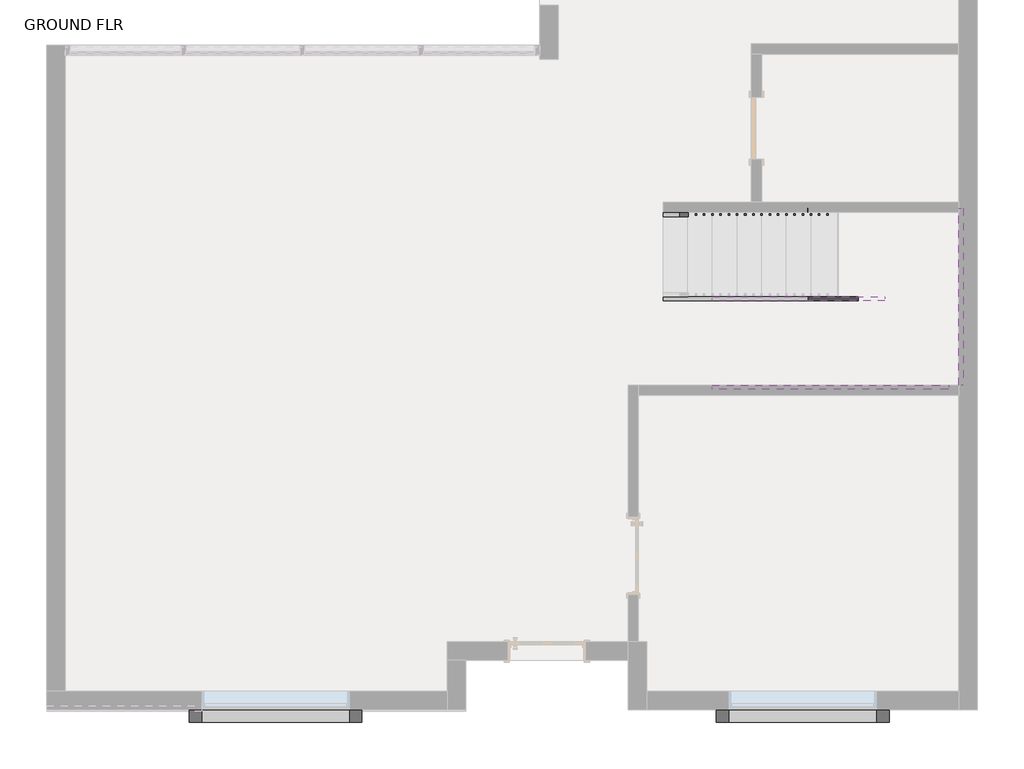
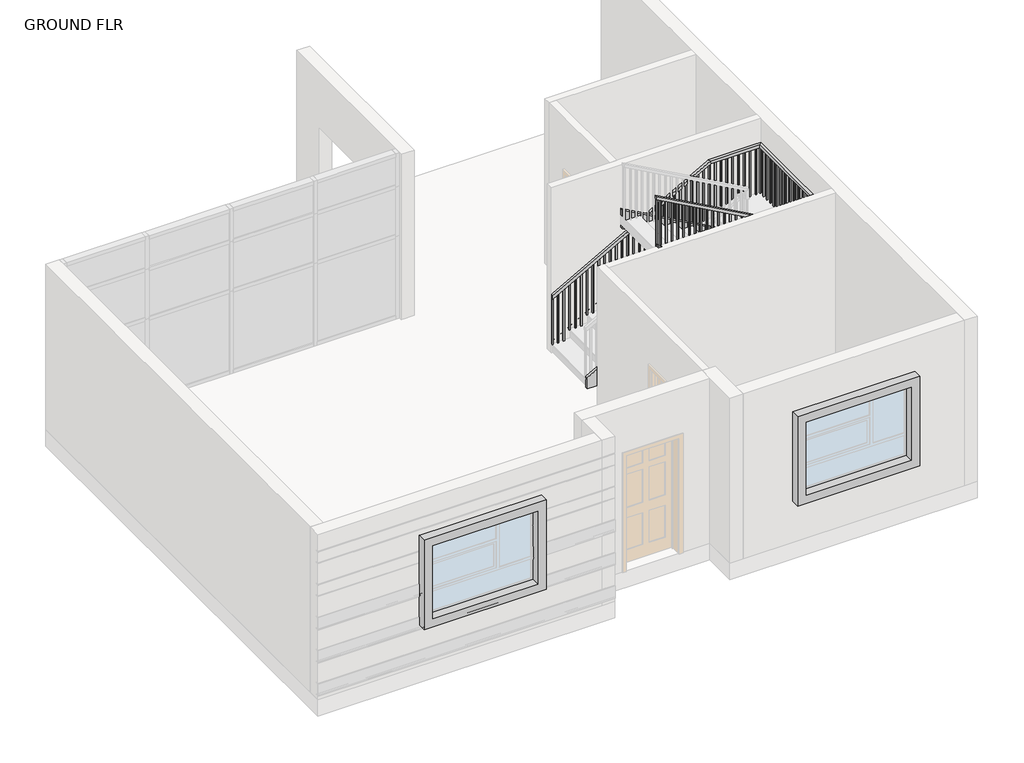
# One storey, part 4 of 4: 5 members, 2 proxies, 1 railing.
"""IFC4 building model written with IfcOpenShell, lengths in millimetres."""

from ifc_helpers import new_model, si_unit, frame, origin, place, context, project, spatial, polyline, outline, extrude, faceted_brep, transform, mapped, element, save
from components import generic_models_3_generic_models_3_1617b94e, generic_models_6_generic_models_3_5dde034f

model = new_model("IFC4")

# Units and contexts
model_context = context("Model", 3, world=origin())
ifc_project = project(units=[si_unit("LENGTHUNIT", "METRE", prefix="MILLI")], contexts=[model_context])

# Site, building, storey
site = spatial("IfcSite", under=ifc_project)
building = spatial("IfcBuilding", under=site)
storey = spatial("IfcBuildingStorey", under=building, Name="GROUND FLR", Elevation=304.8)

# Proxies
placement = place(None, origin())
generic_models_3_generic_models_3_shape = generic_models_3_generic_models_3_1617b94e(model_context)
element("IfcBuildingElementProxy", 1, Name="Generic Models 3 : Generic Models 3", ObjectType="Generic Models 3 : Generic Models 3", at=placement, inside=storey, context=model_context, shape_type="MappedRepresentation", body=[
    mapped(generic_models_3_generic_models_3_shape, transform((0.0, 0.0, 0.0), x_axis=(1.0, 0.0, 0.0), y_axis=(0.0, 1.0, 0.0), z_axis=(0.0, 0.0, 1.0))),
])
generic_models_6_generic_models_3_shape = generic_models_6_generic_models_3_5dde034f(model_context)
element("IfcBuildingElementProxy", 2, Name="Generic Models 6 : Generic Models 3", ObjectType="Generic Models 6 : Generic Models 3", at=placement, inside=storey, context=model_context, shape_type="MappedRepresentation", body=[
    mapped(generic_models_6_generic_models_3_shape, transform((0.0, 0.0, 0.0), x_axis=(1.0, 0.0, 0.0), y_axis=(0.0, 1.0, 0.0), z_axis=(0.0, 0.0, 1.0))),
])

# Members
element("IfcMember", 3, ObjectType="Stringer - 2\" Width", at=placement, inside=storey, context=model_context, shape_type="SweptSolid", body=[
    extrude(outline(polyline([(512.3983948, 1775.9671209), (304.8, 1775.9671209), (304.8, 2029.9116237), (2074.3333333, 5215.0716237), (2074.3333333, 4587.4500103), (512.3983948, 1775.9671209)])), frame((0.0, 3696.9223211, 0.0), z_axis=(0.0, 1.0, 0.0), x_axis=(0.0, 0.0, 1.0)), (0.0, 0.0, 1.0), 50.8),
])
element("IfcMember", 4, ObjectType="Stringer - 2\" Width", at=placement, inside=storey, context=model_context, shape_type="SweptSolid", body=[
    extrude(outline(polyline([(5433.5671209, 3747.7223211), (5484.3671209, 3747.7223211), (5484.3671209, 1563.3223211), (5433.5671209, 1563.3223211), (5433.5671209, 3747.7223211)])), frame((0.0, 0.0, 1769.5333333), z_axis=(0.0, 0.0, 1.0), x_axis=(1.0, 0.0, 0.0)), (0.0, 0.0, 1.0), 304.8),
])
element("IfcMember", 5, ObjectType="Stringer - 2\" Width", at=placement, inside=storey, context=model_context, shape_type="SweptSolid", body=[
    extrude(outline(polyline([(1769.5333333, 5304.3242315), (3391.0650614, 2385.5671209), (3042.3863873, 2385.5671209), (1769.5333333, 4676.7026181), (1769.5333333, 5304.3242315)])), frame((0.0, 1512.5223211, 0.0), z_axis=(0.0, 1.0, 0.0), x_axis=(0.0, 0.0, 1.0)), (0.0, 0.0, 1.0), 50.8),
])
element("IfcMember", 6, ObjectType="Stringer - 2\" Width", at=placement, inside=storey, context=model_context, shape_type="SweptSolid", body=[
    extrude(outline(polyline([(512.3983948, 1775.9671209), (304.8, 1775.9671209), (304.8, 2029.9116237), (1659.4974984, 4468.3671209), (2008.1761726, 4468.3671209), (512.3983948, 1775.9671209)])), frame((0.0, 2604.7223211, 0.0), z_axis=(0.0, 1.0, 0.0), x_axis=(0.0, 0.0, 1.0)), (0.0, 0.0, 1.0), 50.8),
])
element("IfcMember", 7, ObjectType="Stringer - 2\" Width", at=placement, inside=storey, context=model_context, shape_type="SweptSolid", body=[
    extrude(outline(polyline([(1857.053054, 4519.1671209), (2205.7317281, 4519.1671209), (3391.0650614, 2385.5671209), (3042.3863873, 2385.5671209), (1857.053054, 4519.1671209)])), frame((0.0, 2604.7223211, 0.0), z_axis=(0.0, 1.0, 0.0), x_axis=(0.0, 0.0, 1.0)), (0.0, 0.0, 1.0), 50.8),
])

# Railing
element("IfcRailing", 8, ObjectType="Handrail - Rectangular", at=placement, inside=storey, context=model_context, shape_type="SolidModel", body=[
    faceted_brep([(1775.9671209, 3696.9223211, 1388.5333333), (1775.9671209, 3696.9223211, 1330.420221), (1775.9671209, 3646.1223211, 1330.420221), (1775.9671209, 3646.1223211, 1388.5333333), (4519.1671209, 3696.9223211, 2912.5333333), (4532.3307231, 3696.9223211, 2861.7333333), (4532.3307231, 3646.1223211, 2861.7333333), (4519.1671209, 3646.1223211, 2912.5333333), (5433.5671209, 3696.9223211, 2912.5333333), (5433.5671209, 3696.9223211, 2861.7333333), (5382.7671209, 3646.1223211, 2861.7333333), (5382.7671209, 3646.1223211, 2912.5333333), (5433.5671209, 1563.3223211, 2912.5333333), (5433.5671209, 1563.3223211, 2861.7333333), (5382.7671209, 1614.1223211, 2861.7333333), (5382.7671209, 1614.1223211, 2912.5333333), (4823.9671209, 1563.3223211, 2912.5333333), (4810.8035186, 1563.3223211, 2861.7333333), (4810.8035186, 1614.1223211, 2861.7333333), (4823.9671209, 1614.1223211, 2912.5333333), (2385.5671209, 1563.3223211, 4267.2), (2385.5671209, 1614.1223211, 4267.2), (2385.5671209, 1614.1223211, 4209.0868876), (2385.5671209, 1563.3223211, 4209.0868876)], [[[0, 1, 2, 3]], [[1, 0, 4, 5]], [[2, 1, 5, 6]], [[3, 2, 6, 7]], [[0, 3, 7, 4]], [[5, 4, 8, 9]], [[6, 5, 9, 10]], [[7, 6, 10, 11]], [[4, 7, 11, 8]], [[9, 8, 12, 13]], [[10, 9, 13, 14]], [[11, 10, 14, 15]], [[8, 11, 15, 12]], [[13, 12, 16, 17]], [[14, 13, 17, 18]], [[15, 14, 18, 19]], [[12, 15, 19, 16]], [[20, 21, 22, 23]], [[17, 16, 20, 23]], [[18, 17, 23, 22]], [[19, 18, 22, 21]], [[16, 19, 21, 20]]]),
    extrude(outline(polyline([(4172.045221, 2452.2421209), (3183.4666667, 2452.2421209), (3183.4666667, 2471.2921209), (4161.4618876, 2471.2921209), (4172.045221, 2452.2421209)])), frame((0.0, 1579.1973211, 0.0), z_axis=(0.0, 1.0, 0.0), x_axis=(0.0, 0.0, 1.0)), (0.0, 0.0, 1.0), 19.05),
    extrude(outline(polyline([(4115.6007765, 2553.8421209), (3183.4666667, 2553.8421209), (3183.4666667, 2572.8921209), (4105.0174432, 2572.8921209), (4115.6007765, 2553.8421209)])), frame((0.0, 1579.1973211, 0.0), z_axis=(0.0, 1.0, 0.0), x_axis=(0.0, 0.0, 1.0)), (0.0, 0.0, 1.0), 19.05),
    extrude(outline(polyline([(4059.1563321, 2655.4421209), (3183.4666667, 2655.4421209), (3183.4666667, 2674.4921209), (4048.5729988, 2674.4921209), (4059.1563321, 2655.4421209)])), frame((0.0, 1579.1973211, 0.0), z_axis=(0.0, 1.0, 0.0), x_axis=(0.0, 0.0, 1.0)), (0.0, 0.0, 1.0), 19.05),
    extrude(outline(polyline([(4002.7118876, 2757.0421209), (3014.1333333, 2757.0421209), (3014.1333333, 2776.0921209), (3992.1285543, 2776.0921209), (4002.7118876, 2757.0421209)])), frame((0.0, 1579.1973211, 0.0), z_axis=(0.0, 1.0, 0.0), x_axis=(0.0, 0.0, 1.0)), (0.0, 0.0, 1.0), 19.05),
    extrude(outline(polyline([(3946.2674432, 2858.6421209), (3014.1333333, 2858.6421209), (3014.1333333, 2877.6921209), (3935.6841099, 2877.6921209), (3946.2674432, 2858.6421209)])), frame((0.0, 1579.1973211, 0.0), z_axis=(0.0, 1.0, 0.0), x_axis=(0.0, 0.0, 1.0)), (0.0, 0.0, 1.0), 19.05),
    extrude(outline(polyline([(3889.8229988, 2960.2421209), (3014.1333333, 2960.2421209), (3014.1333333, 2979.2921209), (3879.2396654, 2979.2921209), (3889.8229988, 2960.2421209)])), frame((0.0, 1579.1973211, 0.0), z_axis=(0.0, 1.0, 0.0), x_axis=(0.0, 0.0, 1.0)), (0.0, 0.0, 1.0), 19.05),
    extrude(outline(polyline([(3833.3785543, 3061.8421209), (2844.8, 3061.8421209), (2844.8, 3080.8921209), (3822.795221, 3080.8921209), (3833.3785543, 3061.8421209)])), frame((0.0, 1579.1973211, 0.0), z_axis=(0.0, 1.0, 0.0), x_axis=(0.0, 0.0, 1.0)), (0.0, 0.0, 1.0), 19.05),
    extrude(outline(polyline([(3776.9341099, 3163.4421209), (2844.8, 3163.4421209), (2844.8, 3182.4921209), (3766.3507765, 3182.4921209), (3776.9341099, 3163.4421209)])), frame((0.0, 1579.1973211, 0.0), z_axis=(0.0, 1.0, 0.0), x_axis=(0.0, 0.0, 1.0)), (0.0, 0.0, 1.0), 19.05),
    extrude(outline(polyline([(3720.4896654, 3265.0421209), (2844.8, 3265.0421209), (2844.8, 3284.0921209), (3709.9063321, 3284.0921209), (3720.4896654, 3265.0421209)])), frame((0.0, 1579.1973211, 0.0), z_axis=(0.0, 1.0, 0.0), x_axis=(0.0, 0.0, 1.0)), (0.0, 0.0, 1.0), 19.05),
    extrude(outline(polyline([(3664.045221, 3366.6421209), (2675.4666667, 3366.6421209), (2675.4666667, 3385.6921209), (3653.4618876, 3385.6921209), (3664.045221, 3366.6421209)])), frame((0.0, 1579.1973211, 0.0), z_axis=(0.0, 1.0, 0.0), x_axis=(0.0, 0.0, 1.0)), (0.0, 0.0, 1.0), 19.05),
    extrude(outline(polyline([(3607.6007765, 3468.2421209), (2675.4666667, 3468.2421209), (2675.4666667, 3487.2921209), (3597.0174432, 3487.2921209), (3607.6007765, 3468.2421209)])), frame((0.0, 1579.1973211, 0.0), z_axis=(0.0, 1.0, 0.0), x_axis=(0.0, 0.0, 1.0)), (0.0, 0.0, 1.0), 19.05),
    extrude(outline(polyline([(3551.1563321, 3569.8421209), (2675.4666667, 3569.8421209), (2675.4666667, 3588.8921209), (3540.5729988, 3588.8921209), (3551.1563321, 3569.8421209)])), frame((0.0, 1579.1973211, 0.0), z_axis=(0.0, 1.0, 0.0), x_axis=(0.0, 0.0, 1.0)), (0.0, 0.0, 1.0), 19.05),
    extrude(outline(polyline([(3494.7118876, 3671.4421209), (2506.1333333, 3671.4421209), (2506.1333333, 3690.4921209), (3484.1285543, 3690.4921209), (3494.7118876, 3671.4421209)])), frame((0.0, 1579.1973211, 0.0), z_axis=(0.0, 1.0, 0.0), x_axis=(0.0, 0.0, 1.0)), (0.0, 0.0, 1.0), 19.05),
    extrude(outline(polyline([(3438.2674432, 3773.0421209), (2506.1333333, 3773.0421209), (2506.1333333, 3792.0921209), (3427.6841099, 3792.0921209), (3438.2674432, 3773.0421209)])), frame((0.0, 1579.1973211, 0.0), z_axis=(0.0, 1.0, 0.0), x_axis=(0.0, 0.0, 1.0)), (0.0, 0.0, 1.0), 19.05),
    extrude(outline(polyline([(3381.8229988, 3874.6421209), (2506.1333333, 3874.6421209), (2506.1333333, 3893.6921209), (3371.2396654, 3893.6921209), (3381.8229988, 3874.6421209)])), frame((0.0, 1579.1973211, 0.0), z_axis=(0.0, 1.0, 0.0), x_axis=(0.0, 0.0, 1.0)), (0.0, 0.0, 1.0), 19.05),
    extrude(outline(polyline([(3325.3785543, 3976.2421209), (2336.8, 3976.2421209), (2336.8, 3995.2921209), (3314.795221, 3995.2921209), (3325.3785543, 3976.2421209)])), frame((0.0, 1579.1973211, 0.0), z_axis=(0.0, 1.0, 0.0), x_axis=(0.0, 0.0, 1.0)), (0.0, 0.0, 1.0), 19.05),
    extrude(outline(polyline([(3268.9341099, 4077.8421209), (2336.8, 4077.8421209), (2336.8, 4096.8921209), (3258.3507765, 4096.8921209), (3268.9341099, 4077.8421209)])), frame((0.0, 1579.1973211, 0.0), z_axis=(0.0, 1.0, 0.0), x_axis=(0.0, 0.0, 1.0)), (0.0, 0.0, 1.0), 19.05),
    extrude(outline(polyline([(3212.4896654, 4179.4421209), (2336.8, 4179.4421209), (2336.8, 4198.4921209), (3201.9063321, 4198.4921209), (3212.4896654, 4179.4421209)])), frame((0.0, 1579.1973211, 0.0), z_axis=(0.0, 1.0, 0.0), x_axis=(0.0, 0.0, 1.0)), (0.0, 0.0, 1.0), 19.05),
    extrude(outline(polyline([(3156.045221, 4281.0421209), (2167.4666667, 4281.0421209), (2167.4666667, 4300.0921209), (3145.4618876, 4300.0921209), (3156.045221, 4281.0421209)])), frame((0.0, 1579.1973211, 0.0), z_axis=(0.0, 1.0, 0.0), x_axis=(0.0, 0.0, 1.0)), (0.0, 0.0, 1.0), 19.05),
    extrude(outline(polyline([(3099.6007765, 4382.6421209), (2167.4666667, 4382.6421209), (2167.4666667, 4401.6921209), (3089.0174432, 4401.6921209), (3099.6007765, 4382.6421209)])), frame((0.0, 1579.1973211, 0.0), z_axis=(0.0, 1.0, 0.0), x_axis=(0.0, 0.0, 1.0)), (0.0, 0.0, 1.0), 19.05),
    extrude(outline(polyline([(3043.1563321, 4484.2421209), (2167.4666667, 4484.2421209), (2167.4666667, 4503.2921209), (3032.5729988, 4503.2921209), (3043.1563321, 4484.2421209)])), frame((0.0, 1579.1973211, 0.0), z_axis=(0.0, 1.0, 0.0), x_axis=(0.0, 0.0, 1.0)), (0.0, 0.0, 1.0), 19.05),
    extrude(outline(polyline([(2986.7118876, 4585.8421209), (1998.1333333, 4585.8421209), (1998.1333333, 4604.8921209), (2976.1285543, 4604.8921209), (2986.7118876, 4585.8421209)])), frame((0.0, 1579.1973211, 0.0), z_axis=(0.0, 1.0, 0.0), x_axis=(0.0, 0.0, 1.0)), (0.0, 0.0, 1.0), 19.05),
    extrude(outline(polyline([(2930.2674432, 4687.4421209), (1998.1333333, 4687.4421209), (1998.1333333, 4706.4921209), (2919.6841099, 4706.4921209), (2930.2674432, 4687.4421209)])), frame((0.0, 1579.1973211, 0.0), z_axis=(0.0, 1.0, 0.0), x_axis=(0.0, 0.0, 1.0)), (0.0, 0.0, 1.0), 19.05),
    extrude(outline(polyline([(2873.8229988, 4789.0421209), (1998.1333333, 4789.0421209), (1998.1333333, 4808.0921209), (2863.2396654, 4808.0921209), (2873.8229988, 4789.0421209)])), frame((0.0, 1579.1973211, 0.0), z_axis=(0.0, 1.0, 0.0), x_axis=(0.0, 0.0, 1.0)), (0.0, 0.0, 1.0), 19.05),
    extrude(outline(polyline([(4909.6921209, 1579.1973211), (4890.6421209, 1579.1973211), (4890.6421209, 1598.2473211), (4909.6921209, 1598.2473211), (4909.6921209, 1579.1973211)])), frame((0.0, 0.0, 1998.1333333), z_axis=(0.0, 0.0, 1.0), x_axis=(1.0, 0.0, 0.0)), (0.0, 0.0, 1.0), 863.6),
    extrude(outline(polyline([(5011.2921209, 1579.1973211), (4992.2421209, 1579.1973211), (4992.2421209, 1598.2473211), (5011.2921209, 1598.2473211), (5011.2921209, 1579.1973211)])), frame((0.0, 0.0, 1998.1333333), z_axis=(0.0, 0.0, 1.0), x_axis=(1.0, 0.0, 0.0)), (0.0, 0.0, 1.0), 863.6),
    extrude(outline(polyline([(5112.8921209, 1579.1973211), (5093.8421209, 1579.1973211), (5093.8421209, 1598.2473211), (5112.8921209, 1598.2473211), (5112.8921209, 1579.1973211)])), frame((0.0, 0.0, 1998.1333333), z_axis=(0.0, 0.0, 1.0), x_axis=(1.0, 0.0, 0.0)), (0.0, 0.0, 1.0), 863.6),
    extrude(outline(polyline([(5214.4921209, 1579.1973211), (5195.4421209, 1579.1973211), (5195.4421209, 1598.2473211), (5214.4921209, 1598.2473211), (5214.4921209, 1579.1973211)])), frame((0.0, 0.0, 1998.1333333), z_axis=(0.0, 0.0, 1.0), x_axis=(1.0, 0.0, 0.0)), (0.0, 0.0, 1.0), 863.6),
    extrude(outline(polyline([(5316.0921209, 1579.1973211), (5297.0421209, 1579.1973211), (5297.0421209, 1598.2473211), (5316.0921209, 1598.2473211), (5316.0921209, 1579.1973211)])), frame((0.0, 0.0, 1998.1333333), z_axis=(0.0, 0.0, 1.0), x_axis=(1.0, 0.0, 0.0)), (0.0, 0.0, 1.0), 863.6),
    extrude(outline(polyline([(5417.6921209, 1649.0473211), (5417.6921209, 1629.9973211), (5398.6421209, 1629.9973211), (5398.6421209, 1649.0473211), (5417.6921209, 1649.0473211)])), frame((0.0, 0.0, 1998.1333333), z_axis=(0.0, 0.0, 1.0), x_axis=(1.0, 0.0, 0.0)), (0.0, 0.0, 1.0), 863.6),
    extrude(outline(polyline([(5417.6921209, 1750.6473211), (5417.6921209, 1731.5973211), (5398.6421209, 1731.5973211), (5398.6421209, 1750.6473211), (5417.6921209, 1750.6473211)])), frame((0.0, 0.0, 1998.1333333), z_axis=(0.0, 0.0, 1.0), x_axis=(1.0, 0.0, 0.0)), (0.0, 0.0, 1.0), 863.6),
    extrude(outline(polyline([(5417.6921209, 1852.2473211), (5417.6921209, 1833.1973211), (5398.6421209, 1833.1973211), (5398.6421209, 1852.2473211), (5417.6921209, 1852.2473211)])), frame((0.0, 0.0, 1998.1333333), z_axis=(0.0, 0.0, 1.0), x_axis=(1.0, 0.0, 0.0)), (0.0, 0.0, 1.0), 863.6),
    extrude(outline(polyline([(5417.6921209, 1953.8473211), (5417.6921209, 1934.7973211), (5398.6421209, 1934.7973211), (5398.6421209, 1953.8473211), (5417.6921209, 1953.8473211)])), frame((0.0, 0.0, 1998.1333333), z_axis=(0.0, 0.0, 1.0), x_axis=(1.0, 0.0, 0.0)), (0.0, 0.0, 1.0), 863.6),
    extrude(outline(polyline([(5417.6921209, 2055.4473211), (5417.6921209, 2036.3973211), (5398.6421209, 2036.3973211), (5398.6421209, 2055.4473211), (5417.6921209, 2055.4473211)])), frame((0.0, 0.0, 1998.1333333), z_axis=(0.0, 0.0, 1.0), x_axis=(1.0, 0.0, 0.0)), (0.0, 0.0, 1.0), 863.6),
    extrude(outline(polyline([(5417.6921209, 2157.0473211), (5417.6921209, 2137.9973211), (5398.6421209, 2137.9973211), (5398.6421209, 2157.0473211), (5417.6921209, 2157.0473211)])), frame((0.0, 0.0, 1998.1333333), z_axis=(0.0, 0.0, 1.0), x_axis=(1.0, 0.0, 0.0)), (0.0, 0.0, 1.0), 863.6),
    extrude(outline(polyline([(5417.6921209, 2258.6473211), (5417.6921209, 2239.5973211), (5398.6421209, 2239.5973211), (5398.6421209, 2258.6473211), (5417.6921209, 2258.6473211)])), frame((0.0, 0.0, 1998.1333333), z_axis=(0.0, 0.0, 1.0), x_axis=(1.0, 0.0, 0.0)), (0.0, 0.0, 1.0), 863.6),
    extrude(outline(polyline([(5417.6921209, 2360.2473211), (5417.6921209, 2341.1973211), (5398.6421209, 2341.1973211), (5398.6421209, 2360.2473211), (5417.6921209, 2360.2473211)])), frame((0.0, 0.0, 1998.1333333), z_axis=(0.0, 0.0, 1.0), x_axis=(1.0, 0.0, 0.0)), (0.0, 0.0, 1.0), 863.6),
    extrude(outline(polyline([(5417.6921209, 2461.8473211), (5417.6921209, 2442.7973211), (5398.6421209, 2442.7973211), (5398.6421209, 2461.8473211), (5417.6921209, 2461.8473211)])), frame((0.0, 0.0, 1998.1333333), z_axis=(0.0, 0.0, 1.0), x_axis=(1.0, 0.0, 0.0)), (0.0, 0.0, 1.0), 863.6),
    extrude(outline(polyline([(5417.6921209, 2563.4473211), (5417.6921209, 2544.3973211), (5398.6421209, 2544.3973211), (5398.6421209, 2563.4473211), (5417.6921209, 2563.4473211)])), frame((0.0, 0.0, 1998.1333333), z_axis=(0.0, 0.0, 1.0), x_axis=(1.0, 0.0, 0.0)), (0.0, 0.0, 1.0), 863.6),
    extrude(outline(polyline([(5417.6921209, 2665.0473211), (5417.6921209, 2645.9973211), (5398.6421209, 2645.9973211), (5398.6421209, 2665.0473211), (5417.6921209, 2665.0473211)])), frame((0.0, 0.0, 1998.1333333), z_axis=(0.0, 0.0, 1.0), x_axis=(1.0, 0.0, 0.0)), (0.0, 0.0, 1.0), 863.6),
    extrude(outline(polyline([(5417.6921209, 2766.6473211), (5417.6921209, 2747.5973211), (5398.6421209, 2747.5973211), (5398.6421209, 2766.6473211), (5417.6921209, 2766.6473211)])), frame((0.0, 0.0, 1998.1333333), z_axis=(0.0, 0.0, 1.0), x_axis=(1.0, 0.0, 0.0)), (0.0, 0.0, 1.0), 863.6),
    extrude(outline(polyline([(5417.6921209, 2868.2473211), (5417.6921209, 2849.1973211), (5398.6421209, 2849.1973211), (5398.6421209, 2868.2473211), (5417.6921209, 2868.2473211)])), frame((0.0, 0.0, 1998.1333333), z_axis=(0.0, 0.0, 1.0), x_axis=(1.0, 0.0, 0.0)), (0.0, 0.0, 1.0), 863.6),
    extrude(outline(polyline([(5417.6921209, 2969.8473211), (5417.6921209, 2950.7973211), (5398.6421209, 2950.7973211), (5398.6421209, 2969.8473211), (5417.6921209, 2969.8473211)])), frame((0.0, 0.0, 1998.1333333), z_axis=(0.0, 0.0, 1.0), x_axis=(1.0, 0.0, 0.0)), (0.0, 0.0, 1.0), 863.6),
    extrude(outline(polyline([(5417.6921209, 3071.4473211), (5417.6921209, 3052.3973211), (5398.6421209, 3052.3973211), (5398.6421209, 3071.4473211), (5417.6921209, 3071.4473211)])), frame((0.0, 0.0, 1998.1333333), z_axis=(0.0, 0.0, 1.0), x_axis=(1.0, 0.0, 0.0)), (0.0, 0.0, 1.0), 863.6),
    extrude(outline(polyline([(5417.6921209, 3173.0473211), (5417.6921209, 3153.9973211), (5398.6421209, 3153.9973211), (5398.6421209, 3173.0473211), (5417.6921209, 3173.0473211)])), frame((0.0, 0.0, 1998.1333333), z_axis=(0.0, 0.0, 1.0), x_axis=(1.0, 0.0, 0.0)), (0.0, 0.0, 1.0), 863.6),
    extrude(outline(polyline([(5417.6921209, 3274.6473211), (5417.6921209, 3255.5973211), (5398.6421209, 3255.5973211), (5398.6421209, 3274.6473211), (5417.6921209, 3274.6473211)])), frame((0.0, 0.0, 1998.1333333), z_axis=(0.0, 0.0, 1.0), x_axis=(1.0, 0.0, 0.0)), (0.0, 0.0, 1.0), 863.6),
    extrude(outline(polyline([(5417.6921209, 3376.2473211), (5417.6921209, 3357.1973211), (5398.6421209, 3357.1973211), (5398.6421209, 3376.2473211), (5417.6921209, 3376.2473211)])), frame((0.0, 0.0, 1998.1333333), z_axis=(0.0, 0.0, 1.0), x_axis=(1.0, 0.0, 0.0)), (0.0, 0.0, 1.0), 863.6),
    extrude(outline(polyline([(5417.6921209, 3477.8473211), (5417.6921209, 3458.7973211), (5398.6421209, 3458.7973211), (5398.6421209, 3477.8473211), (5417.6921209, 3477.8473211)])), frame((0.0, 0.0, 1998.1333333), z_axis=(0.0, 0.0, 1.0), x_axis=(1.0, 0.0, 0.0)), (0.0, 0.0, 1.0), 863.6),
    extrude(outline(polyline([(5417.6921209, 3579.4473211), (5417.6921209, 3560.3973211), (5398.6421209, 3560.3973211), (5398.6421209, 3579.4473211), (5417.6921209, 3579.4473211)])), frame((0.0, 0.0, 1998.1333333), z_axis=(0.0, 0.0, 1.0), x_axis=(1.0, 0.0, 0.0)), (0.0, 0.0, 1.0), 863.6),
    extrude(outline(polyline([(5322.4421209, 3681.0473211), (5341.4921209, 3681.0473211), (5341.4921209, 3661.9973211), (5322.4421209, 3661.9973211), (5322.4421209, 3681.0473211)])), frame((0.0, 0.0, 1998.1333333), z_axis=(0.0, 0.0, 1.0), x_axis=(1.0, 0.0, 0.0)), (0.0, 0.0, 1.0), 863.6),
    extrude(outline(polyline([(5220.8421209, 3681.0473211), (5239.8921209, 3681.0473211), (5239.8921209, 3661.9973211), (5220.8421209, 3661.9973211), (5220.8421209, 3681.0473211)])), frame((0.0, 0.0, 1998.1333333), z_axis=(0.0, 0.0, 1.0), x_axis=(1.0, 0.0, 0.0)), (0.0, 0.0, 1.0), 863.6),
    extrude(outline(polyline([(5119.2421209, 3681.0473211), (5138.2921209, 3681.0473211), (5138.2921209, 3661.9973211), (5119.2421209, 3661.9973211), (5119.2421209, 3681.0473211)])), frame((0.0, 0.0, 1998.1333333), z_axis=(0.0, 0.0, 1.0), x_axis=(1.0, 0.0, 0.0)), (0.0, 0.0, 1.0), 863.6),
    extrude(outline(polyline([(5017.6421209, 3681.0473211), (5036.6921209, 3681.0473211), (5036.6921209, 3661.9973211), (5017.6421209, 3661.9973211), (5017.6421209, 3681.0473211)])), frame((0.0, 0.0, 1998.1333333), z_axis=(0.0, 0.0, 1.0), x_axis=(1.0, 0.0, 0.0)), (0.0, 0.0, 1.0), 863.6),
    extrude(outline(polyline([(4916.0421209, 3681.0473211), (4935.0921209, 3681.0473211), (4935.0921209, 3661.9973211), (4916.0421209, 3661.9973211), (4916.0421209, 3681.0473211)])), frame((0.0, 0.0, 1998.1333333), z_axis=(0.0, 0.0, 1.0), x_axis=(1.0, 0.0, 0.0)), (0.0, 0.0, 1.0), 863.6),
    extrude(outline(polyline([(4814.4421209, 3681.0473211), (4833.4921209, 3681.0473211), (4833.4921209, 3661.9973211), (4814.4421209, 3661.9973211), (4814.4421209, 3681.0473211)])), frame((0.0, 0.0, 1998.1333333), z_axis=(0.0, 0.0, 1.0), x_axis=(1.0, 0.0, 0.0)), (0.0, 0.0, 1.0), 863.6),
    extrude(outline(polyline([(4712.8421209, 3681.0473211), (4731.8921209, 3681.0473211), (4731.8921209, 3661.9973211), (4712.8421209, 3661.9973211), (4712.8421209, 3681.0473211)])), frame((0.0, 0.0, 1998.1333333), z_axis=(0.0, 0.0, 1.0), x_axis=(1.0, 0.0, 0.0)), (0.0, 0.0, 1.0), 863.6),
    extrude(outline(polyline([(4611.2421209, 3681.0473211), (4630.2921209, 3681.0473211), (4630.2921209, 3661.9973211), (4611.2421209, 3661.9973211), (4611.2421209, 3681.0473211)])), frame((0.0, 0.0, 1998.1333333), z_axis=(0.0, 0.0, 1.0), x_axis=(1.0, 0.0, 0.0)), (0.0, 0.0, 1.0), 863.6),
    extrude(outline(polyline([(2849.1285543, 4509.6421209), (1998.1333333, 4509.6421209), (1998.1333333, 4528.6921209), (2859.7118876, 4528.6921209), (2849.1285543, 4509.6421209)])), frame((0.0, 3661.9973211, 0.0), z_axis=(0.0, 1.0, 0.0), x_axis=(0.0, 0.0, 1.0)), (0.0, 0.0, 1.0), 19.05),
    extrude(outline(polyline([(2792.6841099, 4408.0421209), (1828.8, 4408.0421209), (1828.8, 4427.0921209), (2803.2674432, 4427.0921209), (2792.6841099, 4408.0421209)])), frame((0.0, 3661.9973211, 0.0), z_axis=(0.0, 1.0, 0.0), x_axis=(0.0, 0.0, 1.0)), (0.0, 0.0, 1.0), 19.05),
    extrude(outline(polyline([(2736.2396654, 4306.4421209), (1828.8, 4306.4421209), (1828.8, 4325.4921209), (2746.8229988, 4325.4921209), (2736.2396654, 4306.4421209)])), frame((0.0, 3661.9973211, 0.0), z_axis=(0.0, 1.0, 0.0), x_axis=(0.0, 0.0, 1.0)), (0.0, 0.0, 1.0), 19.05),
    extrude(outline(polyline([(2679.795221, 4204.8421209), (1828.8, 4204.8421209), (1828.8, 4223.8921209), (2690.3785543, 4223.8921209), (2679.795221, 4204.8421209)])), frame((0.0, 3661.9973211, 0.0), z_axis=(0.0, 1.0, 0.0), x_axis=(0.0, 0.0, 1.0)), (0.0, 0.0, 1.0), 19.05),
    extrude(outline(polyline([(2623.3507765, 4103.2421209), (1659.4666667, 4103.2421209), (1659.4666667, 4122.2921209), (2633.9341099, 4122.2921209), (2623.3507765, 4103.2421209)])), frame((0.0, 3661.9973211, 0.0), z_axis=(0.0, 1.0, 0.0), x_axis=(0.0, 0.0, 1.0)), (0.0, 0.0, 1.0), 19.05),
    extrude(outline(polyline([(2566.9063321, 4001.6421209), (1659.4666667, 4001.6421209), (1659.4666667, 4020.6921209), (2577.4896654, 4020.6921209), (2566.9063321, 4001.6421209)])), frame((0.0, 3661.9973211, 0.0), z_axis=(0.0, 1.0, 0.0), x_axis=(0.0, 0.0, 1.0)), (0.0, 0.0, 1.0), 19.05),
    extrude(outline(polyline([(2510.4618876, 3900.0421209), (1659.4666667, 3900.0421209), (1659.4666667, 3919.0921209), (2521.045221, 3919.0921209), (2510.4618876, 3900.0421209)])), frame((0.0, 3661.9973211, 0.0), z_axis=(0.0, 1.0, 0.0), x_axis=(0.0, 0.0, 1.0)), (0.0, 0.0, 1.0), 19.05),
    extrude(outline(polyline([(2454.0174432, 3798.4421209), (1490.1333333, 3798.4421209), (1490.1333333, 3817.4921209), (2464.6007765, 3817.4921209), (2454.0174432, 3798.4421209)])), frame((0.0, 3661.9973211, 0.0), z_axis=(0.0, 1.0, 0.0), x_axis=(0.0, 0.0, 1.0)), (0.0, 0.0, 1.0), 19.05),
    extrude(outline(polyline([(2397.5729988, 3696.8421209), (1490.1333333, 3696.8421209), (1490.1333333, 3715.8921209), (2408.1563321, 3715.8921209), (2397.5729988, 3696.8421209)])), frame((0.0, 3661.9973211, 0.0), z_axis=(0.0, 1.0, 0.0), x_axis=(0.0, 0.0, 1.0)), (0.0, 0.0, 1.0), 19.05),
    extrude(outline(polyline([(2341.1285543, 3595.2421209), (1490.1333333, 3595.2421209), (1490.1333333, 3614.2921209), (2351.7118876, 3614.2921209), (2341.1285543, 3595.2421209)])), frame((0.0, 3661.9973211, 0.0), z_axis=(0.0, 1.0, 0.0), x_axis=(0.0, 0.0, 1.0)), (0.0, 0.0, 1.0), 19.05),
    extrude(outline(polyline([(2284.6841099, 3493.6421209), (1320.8, 3493.6421209), (1320.8, 3512.6921209), (2295.2674432, 3512.6921209), (2284.6841099, 3493.6421209)])), frame((0.0, 3661.9973211, 0.0), z_axis=(0.0, 1.0, 0.0), x_axis=(0.0, 0.0, 1.0)), (0.0, 0.0, 1.0), 19.05),
    extrude(outline(polyline([(2228.2396654, 3392.0421209), (1320.8, 3392.0421209), (1320.8, 3411.0921209), (2238.8229988, 3411.0921209), (2228.2396654, 3392.0421209)])), frame((0.0, 3661.9973211, 0.0), z_axis=(0.0, 1.0, 0.0), x_axis=(0.0, 0.0, 1.0)), (0.0, 0.0, 1.0), 19.05),
    extrude(outline(polyline([(2171.795221, 3290.4421209), (1320.8, 3290.4421209), (1320.8, 3309.4921209), (2182.3785543, 3309.4921209), (2171.795221, 3290.4421209)])), frame((0.0, 3661.9973211, 0.0), z_axis=(0.0, 1.0, 0.0), x_axis=(0.0, 0.0, 1.0)), (0.0, 0.0, 1.0), 19.05),
    extrude(outline(polyline([(2115.3507765, 3188.8421209), (1151.4666667, 3188.8421209), (1151.4666667, 3207.8921209), (2125.9341099, 3207.8921209), (2115.3507765, 3188.8421209)])), frame((0.0, 3661.9973211, 0.0), z_axis=(0.0, 1.0, 0.0), x_axis=(0.0, 0.0, 1.0)), (0.0, 0.0, 1.0), 19.05),
    extrude(outline(polyline([(2058.9063321, 3087.2421209), (1151.4666667, 3087.2421209), (1151.4666667, 3106.2921209), (2069.4896654, 3106.2921209), (2058.9063321, 3087.2421209)])), frame((0.0, 3661.9973211, 0.0), z_axis=(0.0, 1.0, 0.0), x_axis=(0.0, 0.0, 1.0)), (0.0, 0.0, 1.0), 19.05),
    extrude(outline(polyline([(2002.4618876, 2985.6421209), (1151.4666667, 2985.6421209), (1151.4666667, 3004.6921209), (2013.045221, 3004.6921209), (2002.4618876, 2985.6421209)])), frame((0.0, 3661.9973211, 0.0), z_axis=(0.0, 1.0, 0.0), x_axis=(0.0, 0.0, 1.0)), (0.0, 0.0, 1.0), 19.05),
    extrude(outline(polyline([(1946.0174432, 2884.0421209), (982.1333333, 2884.0421209), (982.1333333, 2903.0921209), (1956.6007765, 2903.0921209), (1946.0174432, 2884.0421209)])), frame((0.0, 3661.9973211, 0.0), z_axis=(0.0, 1.0, 0.0), x_axis=(0.0, 0.0, 1.0)), (0.0, 0.0, 1.0), 19.05),
    extrude(outline(polyline([(1889.5729988, 2782.4421209), (982.1333333, 2782.4421209), (982.1333333, 2801.4921209), (1900.1563321, 2801.4921209), (1889.5729988, 2782.4421209)])), frame((0.0, 3661.9973211, 0.0), z_axis=(0.0, 1.0, 0.0), x_axis=(0.0, 0.0, 1.0)), (0.0, 0.0, 1.0), 19.05),
    extrude(outline(polyline([(1833.1285543, 2680.8421209), (982.1333333, 2680.8421209), (982.1333333, 2699.8921209), (1843.7118876, 2699.8921209), (1833.1285543, 2680.8421209)])), frame((0.0, 3661.9973211, 0.0), z_axis=(0.0, 1.0, 0.0), x_axis=(0.0, 0.0, 1.0)), (0.0, 0.0, 1.0), 19.05),
    extrude(outline(polyline([(1776.6841099, 2579.2421209), (812.8, 2579.2421209), (812.8, 2598.2921209), (1787.2674432, 2598.2921209), (1776.6841099, 2579.2421209)])), frame((0.0, 3661.9973211, 0.0), z_axis=(0.0, 1.0, 0.0), x_axis=(0.0, 0.0, 1.0)), (0.0, 0.0, 1.0), 19.05),
    extrude(outline(polyline([(1720.2396654, 2477.6421209), (812.8, 2477.6421209), (812.8, 2496.6921209), (1730.8229988, 2496.6921209), (1720.2396654, 2477.6421209)])), frame((0.0, 3661.9973211, 0.0), z_axis=(0.0, 1.0, 0.0), x_axis=(0.0, 0.0, 1.0)), (0.0, 0.0, 1.0), 19.05),
    extrude(outline(polyline([(1663.795221, 2376.0421209), (812.8, 2376.0421209), (812.8, 2395.0921209), (1674.3785543, 2395.0921209), (1663.795221, 2376.0421209)])), frame((0.0, 3661.9973211, 0.0), z_axis=(0.0, 1.0, 0.0), x_axis=(0.0, 0.0, 1.0)), (0.0, 0.0, 1.0), 19.05),
    extrude(outline(polyline([(1607.3507765, 2274.4421209), (643.4666667, 2274.4421209), (643.4666667, 2293.4921209), (1617.9341099, 2293.4921209), (1607.3507765, 2274.4421209)])), frame((0.0, 3661.9973211, 0.0), z_axis=(0.0, 1.0, 0.0), x_axis=(0.0, 0.0, 1.0)), (0.0, 0.0, 1.0), 19.05),
    extrude(outline(polyline([(1550.9063321, 2172.8421209), (643.4666667, 2172.8421209), (643.4666667, 2191.8921209), (1561.4896654, 2191.8921209), (1550.9063321, 2172.8421209)])), frame((0.0, 3661.9973211, 0.0), z_axis=(0.0, 1.0, 0.0), x_axis=(0.0, 0.0, 1.0)), (0.0, 0.0, 1.0), 19.05),
    extrude(outline(polyline([(1494.4618876, 2071.2421209), (643.4666667, 2071.2421209), (643.4666667, 2090.2921209), (1505.045221, 2090.2921209), (1494.4618876, 2071.2421209)])), frame((0.0, 3661.9973211, 0.0), z_axis=(0.0, 1.0, 0.0), x_axis=(0.0, 0.0, 1.0)), (0.0, 0.0, 1.0), 19.05),
    extrude(outline(polyline([(1438.0174432, 1969.6421209), (474.1333333, 1969.6421209), (474.1333333, 1988.6921209), (1448.6007765, 1988.6921209), (1438.0174432, 1969.6421209)])), frame((0.0, 3661.9973211, 0.0), z_axis=(0.0, 1.0, 0.0), x_axis=(0.0, 0.0, 1.0)), (0.0, 0.0, 1.0), 19.05),
    extrude(outline(polyline([(1381.5729988, 1868.0421209), (474.1333333, 1868.0421209), (474.1333333, 1887.0921209), (1392.1563321, 1887.0921209), (1381.5729988, 1868.0421209)])), frame((0.0, 3661.9973211, 0.0), z_axis=(0.0, 1.0, 0.0), x_axis=(0.0, 0.0, 1.0)), (0.0, 0.0, 1.0), 19.05),
    extrude(outline(polyline([(5417.6921209, 1598.2473211), (5417.6921209, 1579.1973211), (5398.6421209, 1579.1973211), (5398.6421209, 1598.2473211), (5417.6921209, 1598.2473211)])), frame((0.0, 0.0, 1998.1333333), z_axis=(0.0, 0.0, 1.0), x_axis=(1.0, 0.0, 0.0)), (0.0, 0.0, 1.0), 863.6),
    extrude(outline(polyline([(5398.6421209, 3681.0473211), (5417.6921209, 3681.0473211), (5417.6921209, 3661.9973211), (5398.6421209, 3661.9973211), (5398.6421209, 3681.0473211)])), frame((0.0, 0.0, 1998.1333333), z_axis=(0.0, 0.0, 1.0), x_axis=(1.0, 0.0, 0.0)), (0.0, 0.0, 1.0), 863.6),
    extrude(outline(polyline([(4209.0868876, 2385.5671209), (3183.4666667, 2385.5671209), (3183.4666667, 2404.6171209), (4198.5035543, 2404.6171209), (4209.0868876, 2385.5671209)])), frame((0.0, 1579.1973211, 0.0), z_axis=(0.0, 1.0, 0.0), x_axis=(0.0, 0.0, 1.0)), (0.0, 0.0, 1.0), 19.05),
    extrude(outline(polyline([(1330.420221, 1775.9671209), (474.1333333, 1775.9671209), (474.1333333, 1795.0171209), (1341.0035543, 1795.0171209), (1330.420221, 1775.9671209)])), frame((0.0, 3661.9973211, 0.0), z_axis=(0.0, 1.0, 0.0), x_axis=(0.0, 0.0, 1.0)), (0.0, 0.0, 1.0), 19.05),
])

save(model, "model.ifc")

# Revit data of these elements
# Type "Handrail - Rectangular"
#   Assembly Code = "C2010400"
#   built-in parameter 1008612 = 0.0416667 (stored number, unit not read)
#   built-in parameter 1008611 = 0.0416667 (stored number, unit not read)
#   built-in parameter 1008609 = 0.333333 (stored number, unit not read)
#   built-in parameter 1008604 = 0.166667 (stored number, unit not read)
#   built-in parameter 1008603 = 0.166667 (stored number, unit not read)
#   Railing Height = 3' - 0"
#   built-in parameter 1008630 = 2
#   built-in parameter 1008610 = 2
#   built-in parameter 1008618 = Baluster - Square : 3/4"
# Element 1 (IfcBuildingElementProxy, "Generic Models 3 : Generic Models 3")
#   Phase Created = New Construction
#   Materials on its faces: "WALNUT WOOD COLOUR 5\""
# Element 2 (IfcBuildingElementProxy, "Generic Models 6 : Generic Models 3")
#   Phase Created = New Construction
#   Materials on its faces: "WALNUT WOOD COLOUR 5\""
# Elements 3, 4, 5, 6, 7 (IfcMember, "Stringer - 2\" Width")
#   Phase Created = New Construction
# Element 8 (IfcRailing, "Handrail - Rectangular")
#   Phase Created = New Construction
# Materials
#   "WALNUT WOOD COLOUR 5\"": class "Generic", colour RGB 120 120 120, transparency 0, Cost = 0
